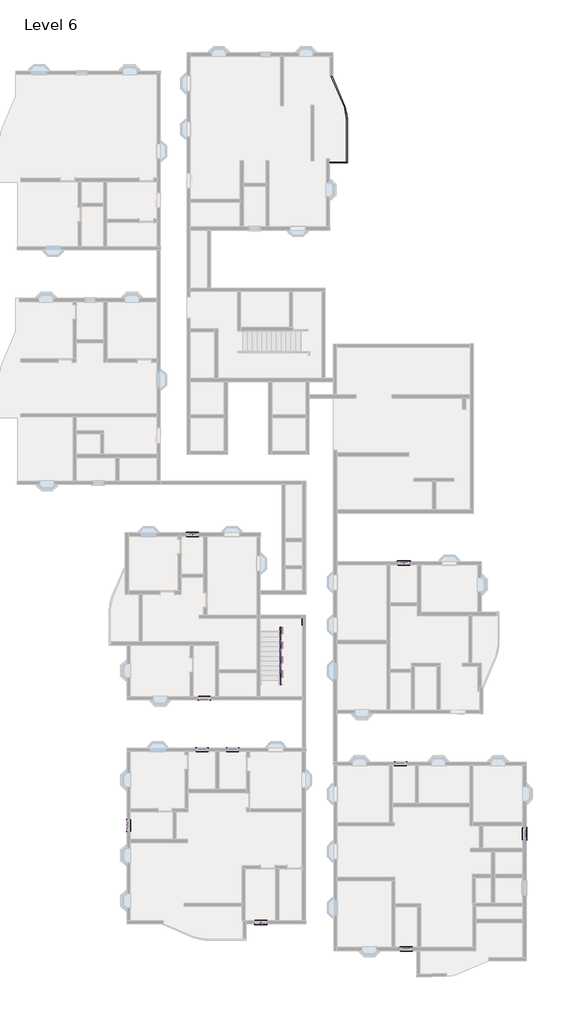
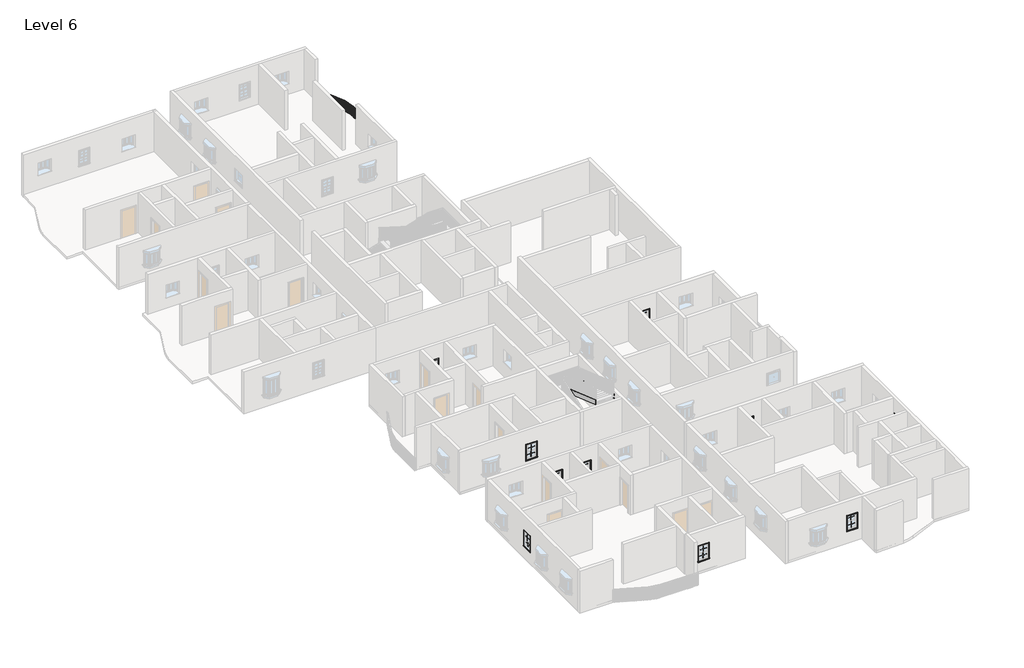
# One storey, part 13 of 14: 40 proxies, 6 members, 1 railing.
"""IFC4 building model written with IfcOpenShell, lengths in millimetres."""

from ifc_helpers import new_model, si_unit, frame, origin, place, context, project, spatial, polyline, circle_curve, outline, extrude, transform, mapped, element, save
from ifc_brep_helpers import plane_surface, cylinder_surface, revolved_surface, advanced_brep
from components import muntin_pattern_2x2_muntin_pattern_2x2_c35c595f, trim_window_exterior_flat_with_sill_e38017c9, trim_window_interior_flat_picture_frame_d728ed12

model = new_model("IFC4")

# Units and contexts
model_context = context("Model", 3, world=origin())
ifc_project = project(units=[si_unit("LENGTHUNIT", "METRE", prefix="MILLI")], contexts=[model_context])

# Site, building, storey
site = spatial("IfcSite", under=ifc_project)
building = spatial("IfcBuilding", under=site)
storey = spatial("IfcBuildingStorey", under=building, Name="Level 6", Elevation=15240.0)

# Proxies
placement = place(None, origin())
muntin_pattern_2x2_muntin_pattern_2x2_shape = muntin_pattern_2x2_muntin_pattern_2x2_c35c595f(model_context)
element("IfcBuildingElementProxy", 1, Name="Muntin Pattern_2x2 : Muntin Pattern_2x2", ObjectType="Muntin Pattern_2x2 : Muntin Pattern_2x2", at=placement, inside=storey, context=model_context, shape_type="MappedRepresentation", body=[
    mapped(muntin_pattern_2x2_muntin_pattern_2x2_shape, transform((-8150.287215, -357.5666506, 16710.025), x_axis=(1.0, 0.0, 0.0), y_axis=(0.0, 1.0, 0.0), z_axis=(0.0, 0.0, 1.0))),
])
element("IfcBuildingElementProxy", 2, Name="Muntin Pattern_2x2 : Muntin Pattern_2x2", ObjectType="Muntin Pattern_2x2 : Muntin Pattern_2x2", at=placement, inside=storey, context=model_context, shape_type="MappedRepresentation", body=[
    mapped(muntin_pattern_2x2_muntin_pattern_2x2_shape, transform((-8150.287215, -402.0166506, 16230.6), x_axis=(1.0, 0.0, 0.0), y_axis=(0.0, 1.0, 0.0), z_axis=(0.0, 0.0, 1.0))),
])
element("IfcBuildingElementProxy", 3, Name="Muntin Pattern_2x2 : Muntin Pattern_2x2", ObjectType="Muntin Pattern_2x2 : Muntin Pattern_2x2", at=placement, inside=storey, context=model_context, shape_type="MappedRepresentation", body=[
    mapped(muntin_pattern_2x2_muntin_pattern_2x2_shape, transform((-7397.812215, -10854.1166506, 16710.025), x_axis=(-1.0, 0.0, 0.0), y_axis=(0.0, -1.0, 0.0), z_axis=(0.0, 0.0, 1.0))),
])
element("IfcBuildingElementProxy", 4, Name="Muntin Pattern_2x2 : Muntin Pattern_2x2", ObjectType="Muntin Pattern_2x2 : Muntin Pattern_2x2", at=placement, inside=storey, context=model_context, shape_type="MappedRepresentation", body=[
    mapped(muntin_pattern_2x2_muntin_pattern_2x2_shape, transform((-7397.812215, -10809.6666506, 16230.6), x_axis=(-1.0, 0.0, 0.0), y_axis=(0.0, -1.0, 0.0), z_axis=(0.0, 0.0, 1.0))),
])
element("IfcBuildingElementProxy", 5, Name="Muntin Pattern_2x2 : Muntin Pattern_2x2", ObjectType="Muntin Pattern_2x2 : Muntin Pattern_2x2", at=placement, inside=storey, context=model_context, shape_type="MappedRepresentation", body=[
    mapped(muntin_pattern_2x2_muntin_pattern_2x2_shape, transform((-7540.687215, -13997.3666506, 16710.025), x_axis=(1.0, 0.0, 0.0), y_axis=(0.0, 1.0, 0.0), z_axis=(0.0, 0.0, 1.0))),
])
element("IfcBuildingElementProxy", 6, Name="Muntin Pattern_2x2 : Muntin Pattern_2x2", ObjectType="Muntin Pattern_2x2 : Muntin Pattern_2x2", at=placement, inside=storey, context=model_context, shape_type="MappedRepresentation", body=[
    mapped(muntin_pattern_2x2_muntin_pattern_2x2_shape, transform((-7540.687215, -14041.8166506, 16230.6), x_axis=(1.0, 0.0, 0.0), y_axis=(0.0, 1.0, 0.0), z_axis=(0.0, 0.0, 1.0))),
])
element("IfcBuildingElementProxy", 7, Name="Muntin Pattern_2x2 : Muntin Pattern_2x2", ObjectType="Muntin Pattern_2x2 : Muntin Pattern_2x2", at=placement, inside=storey, context=model_context, shape_type="MappedRepresentation", body=[
    mapped(muntin_pattern_2x2_muntin_pattern_2x2_shape, transform((-5597.587215, -13997.3666506, 16710.025), x_axis=(1.0, 0.0, 0.0), y_axis=(0.0, 1.0, 0.0), z_axis=(0.0, 0.0, 1.0))),
])
element("IfcBuildingElementProxy", 8, Name="Muntin Pattern_2x2 : Muntin Pattern_2x2", ObjectType="Muntin Pattern_2x2 : Muntin Pattern_2x2", at=placement, inside=storey, context=model_context, shape_type="MappedRepresentation", body=[
    mapped(muntin_pattern_2x2_muntin_pattern_2x2_shape, transform((-5597.587215, -14041.8166506, 16230.6), x_axis=(1.0, 0.0, 0.0), y_axis=(0.0, 1.0, 0.0), z_axis=(0.0, 0.0, 1.0))),
])
element("IfcBuildingElementProxy", 9, Name="Muntin Pattern_2x2 : Muntin Pattern_2x2", ObjectType="Muntin Pattern_2x2 : Muntin Pattern_2x2", at=placement, inside=storey, context=model_context, shape_type="MappedRepresentation", body=[
    mapped(muntin_pattern_2x2_muntin_pattern_2x2_shape, transform((-12255.562215, -18863.6994419, 16710.025), x_axis=(0.0, 1.0, 0.0), y_axis=(-1.0, 0.0, 0.0), z_axis=(0.0, 0.0, 1.0))),
])
element("IfcBuildingElementProxy", 10, Name="Muntin Pattern_2x2 : Muntin Pattern_2x2", ObjectType="Muntin Pattern_2x2 : Muntin Pattern_2x2", at=placement, inside=storey, context=model_context, shape_type="MappedRepresentation", body=[
    mapped(muntin_pattern_2x2_muntin_pattern_2x2_shape, transform((-12211.112215, -18863.6994419, 16230.6), x_axis=(0.0, 1.0, 0.0), y_axis=(-1.0, 0.0, 0.0), z_axis=(0.0, 0.0, 1.0))),
])
element("IfcBuildingElementProxy", 11, Name="Muntin Pattern_2x2 : Muntin Pattern_2x2", ObjectType="Muntin Pattern_2x2 : Muntin Pattern_2x2", at=placement, inside=storey, context=model_context, shape_type="MappedRepresentation", body=[
    mapped(muntin_pattern_2x2_muntin_pattern_2x2_shape, transform((-3806.2891351, -25065.4166506, 16710.025), x_axis=(-1.0, 0.0, 0.0), y_axis=(0.0, -1.0, 0.0), z_axis=(0.0, 0.0, 1.0))),
])
element("IfcBuildingElementProxy", 12, Name="Muntin Pattern_2x2 : Muntin Pattern_2x2", ObjectType="Muntin Pattern_2x2 : Muntin Pattern_2x2", at=placement, inside=storey, context=model_context, shape_type="MappedRepresentation", body=[
    mapped(muntin_pattern_2x2_muntin_pattern_2x2_shape, transform((-3806.2891351, -25020.9666506, 16230.6), x_axis=(-1.0, 0.0, 0.0), y_axis=(0.0, -1.0, 0.0), z_axis=(0.0, 0.0, 1.0))),
])
element("IfcBuildingElementProxy", 13, Name="Muntin Pattern_2x2 : Muntin Pattern_2x2", ObjectType="Muntin Pattern_2x2 : Muntin Pattern_2x2", at=placement, inside=storey, context=model_context, shape_type="MappedRepresentation", body=[
    mapped(muntin_pattern_2x2_muntin_pattern_2x2_shape, transform((5410.0380523, -26615.6292694, 16710.025), x_axis=(1.0, 0.0, 0.0), y_axis=(0.0, 1.0, 0.0), z_axis=(0.0, 0.0, 1.0))),
])
element("IfcBuildingElementProxy", 14, Name="Muntin Pattern_2x2 : Muntin Pattern_2x2", ObjectType="Muntin Pattern_2x2 : Muntin Pattern_2x2", at=placement, inside=storey, context=model_context, shape_type="MappedRepresentation", body=[
    mapped(muntin_pattern_2x2_muntin_pattern_2x2_shape, transform((5410.0380523, -26660.0792694, 16230.6), x_axis=(1.0, 0.0, 0.0), y_axis=(0.0, 1.0, 0.0), z_axis=(0.0, 0.0, 1.0))),
])
element("IfcBuildingElementProxy", 15, Name="Muntin Pattern_2x2 : Muntin Pattern_2x2", ObjectType="Muntin Pattern_2x2 : Muntin Pattern_2x2", at=placement, inside=storey, context=model_context, shape_type="MappedRepresentation", body=[
    mapped(muntin_pattern_2x2_muntin_pattern_2x2_shape, transform((12982.4130523, -19379.8042694, 16710.025), x_axis=(0.0, -1.0, 0.0), y_axis=(1.0, 0.0, 0.0), z_axis=(0.0, 0.0, 1.0))),
])
element("IfcBuildingElementProxy", 16, Name="Muntin Pattern_2x2 : Muntin Pattern_2x2", ObjectType="Muntin Pattern_2x2 : Muntin Pattern_2x2", at=placement, inside=storey, context=model_context, shape_type="MappedRepresentation", body=[
    mapped(muntin_pattern_2x2_muntin_pattern_2x2_shape, transform((12937.9630523, -19379.8042694, 16230.6), x_axis=(0.0, -1.0, 0.0), y_axis=(1.0, 0.0, 0.0), z_axis=(0.0, 0.0, 1.0))),
])
element("IfcBuildingElementProxy", 17, Name="Muntin Pattern_2x2 : Muntin Pattern_2x2", ObjectType="Muntin Pattern_2x2 : Muntin Pattern_2x2", at=placement, inside=storey, context=model_context, shape_type="MappedRepresentation", body=[
    mapped(muntin_pattern_2x2_muntin_pattern_2x2_shape, transform((5048.0880523, -14880.8292694, 16710.025), x_axis=(1.0, 0.0, 0.0), y_axis=(0.0, 1.0, 0.0), z_axis=(0.0, 0.0, 1.0))),
])
element("IfcBuildingElementProxy", 18, Name="Muntin Pattern_2x2 : Muntin Pattern_2x2", ObjectType="Muntin Pattern_2x2 : Muntin Pattern_2x2", at=placement, inside=storey, context=model_context, shape_type="MappedRepresentation", body=[
    mapped(muntin_pattern_2x2_muntin_pattern_2x2_shape, transform((5048.0880523, -14925.2792694, 16230.6), x_axis=(1.0, 0.0, 0.0), y_axis=(0.0, 1.0, 0.0), z_axis=(0.0, 0.0, 1.0))),
])
element("IfcBuildingElementProxy", 19, Name="Muntin Pattern_2x2 : Muntin Pattern_2x2", ObjectType="Muntin Pattern_2x2 : Muntin Pattern_2x2", at=placement, inside=storey, context=model_context, shape_type="MappedRepresentation", body=[
    mapped(muntin_pattern_2x2_muntin_pattern_2x2_shape, transform((5257.6380523, -2168.1292694, 16710.025), x_axis=(1.0, 0.0, 0.0), y_axis=(0.0, 1.0, 0.0), z_axis=(0.0, 0.0, 1.0))),
])
element("IfcBuildingElementProxy", 20, Name="Muntin Pattern_2x2 : Muntin Pattern_2x2", ObjectType="Muntin Pattern_2x2 : Muntin Pattern_2x2", at=placement, inside=storey, context=model_context, shape_type="MappedRepresentation", body=[
    mapped(muntin_pattern_2x2_muntin_pattern_2x2_shape, transform((5257.6380523, -2212.5792694, 16230.6), x_axis=(1.0, 0.0, 0.0), y_axis=(0.0, 1.0, 0.0), z_axis=(0.0, 0.0, 1.0))),
])
trim_window_exterior_flat_with_sill_shape = trim_window_exterior_flat_with_sill_e38017c9(model_context)
element("IfcBuildingElementProxy", 21, Name="Trim-Window-Exterior-Flat : with Sill", ObjectType="Trim-Window-Exterior-Flat : with Sill", at=placement, inside=storey, context=model_context, shape_type="MappedRepresentation", body=[
    mapped(trim_window_exterior_flat_with_sill_shape, transform((-8150.287215, -322.6416506, 17221.2), x_axis=(-1.0, 0.0, 0.0), y_axis=(0.0, 0.0, 1.0), z_axis=(0.0, 1.0, 0.0))),
])
element("IfcBuildingElementProxy", 22, Name="Trim-Window-Exterior-Flat : with Sill", ObjectType="Trim-Window-Exterior-Flat : with Sill", at=placement, inside=storey, context=model_context, shape_type="MappedRepresentation", body=[
    mapped(trim_window_exterior_flat_with_sill_shape, transform((-7397.812215, -10889.0416506, 17221.2), x_axis=(1.0, 0.0, 0.0), y_axis=(0.0, 0.0, 1.0), z_axis=(0.0, -1.0, 0.0))),
])
element("IfcBuildingElementProxy", 23, Name="Trim-Window-Exterior-Flat : with Sill", ObjectType="Trim-Window-Exterior-Flat : with Sill", at=placement, inside=storey, context=model_context, shape_type="MappedRepresentation", body=[
    mapped(trim_window_exterior_flat_with_sill_shape, transform((-7540.687215, -13962.4416506, 17221.2), x_axis=(-1.0, 0.0, 0.0), y_axis=(0.0, 0.0, 1.0), z_axis=(0.0, 1.0, 0.0))),
])
element("IfcBuildingElementProxy", 24, Name="Trim-Window-Exterior-Flat : with Sill", ObjectType="Trim-Window-Exterior-Flat : with Sill", at=placement, inside=storey, context=model_context, shape_type="MappedRepresentation", body=[
    mapped(trim_window_exterior_flat_with_sill_shape, transform((-5597.587215, -13962.4416506, 17221.2), x_axis=(-1.0, 0.0, 0.0), y_axis=(0.0, 0.0, 1.0), z_axis=(0.0, 1.0, 0.0))),
])
element("IfcBuildingElementProxy", 25, Name="Trim-Window-Exterior-Flat : with Sill", ObjectType="Trim-Window-Exterior-Flat : with Sill", at=placement, inside=storey, context=model_context, shape_type="MappedRepresentation", body=[
    mapped(trim_window_exterior_flat_with_sill_shape, transform((-12290.487215, -18863.6994419, 17221.2), x_axis=(0.0, -1.0, 0.0), y_axis=(0.0, 0.0, 1.0), z_axis=(-1.0, 0.0, 0.0))),
])
element("IfcBuildingElementProxy", 26, Name="Trim-Window-Exterior-Flat : with Sill", ObjectType="Trim-Window-Exterior-Flat : with Sill", at=placement, inside=storey, context=model_context, shape_type="MappedRepresentation", body=[
    mapped(trim_window_exterior_flat_with_sill_shape, transform((-3806.2891351, -25100.3416506, 17221.2), x_axis=(1.0, 0.0, 0.0), y_axis=(0.0, 0.0, 1.0), z_axis=(0.0, -1.0, 0.0))),
])
element("IfcBuildingElementProxy", 27, Name="Trim-Window-Exterior-Flat : with Sill", ObjectType="Trim-Window-Exterior-Flat : with Sill", at=placement, inside=storey, context=model_context, shape_type="MappedRepresentation", body=[
    mapped(trim_window_exterior_flat_with_sill_shape, transform((5410.0380523, -26580.7042694, 17221.2), x_axis=(-1.0, 0.0, 0.0), y_axis=(0.0, 0.0, 1.0), z_axis=(0.0, 1.0, 0.0))),
])
element("IfcBuildingElementProxy", 28, Name="Trim-Window-Exterior-Flat : with Sill", ObjectType="Trim-Window-Exterior-Flat : with Sill", at=placement, inside=storey, context=model_context, shape_type="MappedRepresentation", body=[
    mapped(trim_window_exterior_flat_with_sill_shape, transform((13017.3380523, -19379.8042694, 17221.2), x_axis=(0.0, 1.0, 0.0), y_axis=(0.0, 0.0, 1.0), z_axis=(1.0, 0.0, 0.0))),
])
element("IfcBuildingElementProxy", 29, Name="Trim-Window-Exterior-Flat : with Sill", ObjectType="Trim-Window-Exterior-Flat : with Sill", at=placement, inside=storey, context=model_context, shape_type="MappedRepresentation", body=[
    mapped(trim_window_exterior_flat_with_sill_shape, transform((5048.0880523, -14845.9042694, 17221.2), x_axis=(-1.0, 0.0, 0.0), y_axis=(0.0, 0.0, 1.0), z_axis=(0.0, 1.0, 0.0))),
])
element("IfcBuildingElementProxy", 30, Name="Trim-Window-Exterior-Flat : with Sill", ObjectType="Trim-Window-Exterior-Flat : with Sill", at=placement, inside=storey, context=model_context, shape_type="MappedRepresentation", body=[
    mapped(trim_window_exterior_flat_with_sill_shape, transform((5257.6380523, -2133.2042694, 17221.2), x_axis=(-1.0, 0.0, 0.0), y_axis=(0.0, 0.0, 1.0), z_axis=(0.0, 1.0, 0.0))),
])
trim_window_interior_flat_picture_frame_shape = trim_window_interior_flat_picture_frame_d728ed12(model_context)
element("IfcBuildingElementProxy", 31, Name="Trim-Window-Interior-Flat : Picture Frame", ObjectType="Trim-Window-Interior-Flat : Picture Frame", at=placement, inside=storey, context=model_context, shape_type="MappedRepresentation", body=[
    mapped(trim_window_interior_flat_picture_frame_shape, transform((-8150.287215, -525.8416506, 17221.2), x_axis=(1.0, 0.0, 0.0), y_axis=(0.0, 0.0, 1.0), z_axis=(0.0, -1.0, 0.0))),
])
element("IfcBuildingElementProxy", 32, Name="Trim-Window-Interior-Flat : Picture Frame", ObjectType="Trim-Window-Interior-Flat : Picture Frame", at=placement, inside=storey, context=model_context, shape_type="MappedRepresentation", body=[
    mapped(trim_window_interior_flat_picture_frame_shape, transform((-7397.812215, -10685.8416506, 17221.2), x_axis=(-1.0, 0.0, 0.0), y_axis=(0.0, 0.0, 1.0), z_axis=(0.0, 1.0, 0.0))),
])
element("IfcBuildingElementProxy", 33, Name="Trim-Window-Interior-Flat : Picture Frame", ObjectType="Trim-Window-Interior-Flat : Picture Frame", at=placement, inside=storey, context=model_context, shape_type="MappedRepresentation", body=[
    mapped(trim_window_interior_flat_picture_frame_shape, transform((-7540.687215, -14165.6416506, 17221.2), x_axis=(1.0, 0.0, 0.0), y_axis=(0.0, 0.0, 1.0), z_axis=(0.0, -1.0, 0.0))),
])
element("IfcBuildingElementProxy", 34, Name="Trim-Window-Interior-Flat : Picture Frame", ObjectType="Trim-Window-Interior-Flat : Picture Frame", at=placement, inside=storey, context=model_context, shape_type="MappedRepresentation", body=[
    mapped(trim_window_interior_flat_picture_frame_shape, transform((-5597.587215, -14165.6416506, 17221.2), x_axis=(1.0, 0.0, 0.0), y_axis=(0.0, 0.0, 1.0), z_axis=(0.0, -1.0, 0.0))),
])
element("IfcBuildingElementProxy", 35, Name="Trim-Window-Interior-Flat : Picture Frame", ObjectType="Trim-Window-Interior-Flat : Picture Frame", at=placement, inside=storey, context=model_context, shape_type="MappedRepresentation", body=[
    mapped(trim_window_interior_flat_picture_frame_shape, transform((-12087.287215, -18863.6994419, 17221.2), x_axis=(0.0, 1.0, 0.0), y_axis=(0.0, 0.0, 1.0), z_axis=(1.0, 0.0, 0.0))),
])
element("IfcBuildingElementProxy", 36, Name="Trim-Window-Interior-Flat : Picture Frame", ObjectType="Trim-Window-Interior-Flat : Picture Frame", at=placement, inside=storey, context=model_context, shape_type="MappedRepresentation", body=[
    mapped(trim_window_interior_flat_picture_frame_shape, transform((-3806.2891351, -24897.1416506, 17221.2), x_axis=(-1.0, 0.0, 0.0), y_axis=(0.0, 0.0, 1.0), z_axis=(0.0, 1.0, 0.0))),
])
element("IfcBuildingElementProxy", 37, Name="Trim-Window-Interior-Flat : Picture Frame", ObjectType="Trim-Window-Interior-Flat : Picture Frame", at=placement, inside=storey, context=model_context, shape_type="MappedRepresentation", body=[
    mapped(trim_window_interior_flat_picture_frame_shape, transform((5410.0380523, -26783.9042694, 17221.2), x_axis=(1.0, 0.0, 0.0), y_axis=(0.0, 0.0, 1.0), z_axis=(0.0, -1.0, 0.0))),
])
element("IfcBuildingElementProxy", 38, Name="Trim-Window-Interior-Flat : Picture Frame", ObjectType="Trim-Window-Interior-Flat : Picture Frame", at=placement, inside=storey, context=model_context, shape_type="MappedRepresentation", body=[
    mapped(trim_window_interior_flat_picture_frame_shape, transform((12814.1380523, -19379.8042694, 17221.2), x_axis=(0.0, -1.0, 0.0), y_axis=(0.0, 0.0, 1.0), z_axis=(-1.0, 0.0, 0.0))),
])
element("IfcBuildingElementProxy", 39, Name="Trim-Window-Interior-Flat : Picture Frame", ObjectType="Trim-Window-Interior-Flat : Picture Frame", at=placement, inside=storey, context=model_context, shape_type="MappedRepresentation", body=[
    mapped(trim_window_interior_flat_picture_frame_shape, transform((5048.0880523, -15049.1042694, 17221.2), x_axis=(1.0, 0.0, 0.0), y_axis=(0.0, 0.0, 1.0), z_axis=(0.0, -1.0, 0.0))),
])
element("IfcBuildingElementProxy", 40, Name="Trim-Window-Interior-Flat : Picture Frame", ObjectType="Trim-Window-Interior-Flat : Picture Frame", at=placement, inside=storey, context=model_context, shape_type="MappedRepresentation", body=[
    mapped(trim_window_interior_flat_picture_frame_shape, transform((5257.6380523, -2336.4042694, 17221.2), x_axis=(1.0, 0.0, 0.0), y_axis=(0.0, 0.0, 1.0), z_axis=(0.0, -1.0, 0.0))),
])

# Members
element("IfcMember", 41, ObjectType="Stringer - 2\" Width", at=placement, inside=storey, context=model_context, shape_type="SweptSolid", body=[
    extrude(outline(polyline([(-9955.5916506, 15240.0), (-9955.5916506, 15431.3592169), (-6325.8738327, 16687.8), (-5713.7916506, 16687.8), (-5713.7916506, 16577.1301656), (-9576.612129, 15240.0), (-9955.5916506, 15240.0)])), frame((-3908.487215, 0.0, 0.0), z_axis=(1.0, 0.0, 0.0), x_axis=(0.0, 1.0, 0.0)), (0.0, 0.0, 1.0), 50.8),
])
element("IfcMember", 42, ObjectType="Stringer - 2\" Width", at=placement, inside=storey, context=model_context, shape_type="SweptSolid", body=[
    extrude(outline(polyline([(-3908.487215, -5713.7916506), (-3908.487215, -5662.9916506), (-1190.687215, -5662.9916506), (-1190.687215, -5713.7916506), (-3908.487215, -5713.7916506)])), frame((0.0, 0.0, 16383.0), z_axis=(0.0, 0.0, 1.0), x_axis=(1.0, 0.0, 0.0)), (0.0, 0.0, 1.0), 304.8),
])
element("IfcMember", 43, ObjectType="Stringer - 2\" Width", at=placement, inside=storey, context=model_context, shape_type="SweptSolid", body=[
    extrude(outline(polyline([(-5662.9916506, 16587.5476784), (-5662.9916506, 16383.0), (-6003.8711722, 16383.0), (-9949.2416506, 17748.7051656), (-9949.2416506, 18071.2496015), (-5662.9916506, 16587.5476784)])), frame((-1190.687215, 0.0, 0.0), z_axis=(1.0, 0.0, 0.0), x_axis=(0.0, 1.0, 0.0)), (0.0, 0.0, 1.0), 50.8),
])
element("IfcMember", 44, ObjectType="Stringer - 2\" Width", at=placement, inside=storey, context=model_context, shape_type="SweptSolid", body=[
    extrude(outline(polyline([(-9955.5916506, 15240.0), (-9955.5916506, 15431.3592169), (-6342.4416506, 16682.0649861), (-6342.4416506, 16359.5205502), (-9576.612129, 15240.0), (-9955.5916506, 15240.0)])), frame((-2593.7381751, 0.0, 0.0), z_axis=(1.0, 0.0, 0.0), x_axis=(0.0, 1.0, 0.0)), (0.0, 0.0, 1.0), 50.8),
])
element("IfcMember", 45, ObjectType="Stringer - 2\" Width", at=placement, inside=storey, context=model_context, shape_type="SweptSolid", body=[
    extrude(outline(polyline([(-2593.7381751, -6342.4416506), (-2593.7381751, -6291.6416506), (-2492.1381751, -6291.6416506), (-2492.1381751, -6342.4416506), (-2593.7381751, -6342.4416506)])), frame((0.0, 0.0, 16383.0), z_axis=(0.0, 0.0, 1.0), x_axis=(1.0, 0.0, 0.0)), (0.0, 0.0, 1.0), 304.8),
])
element("IfcMember", 46, ObjectType="Stringer - 2\" Width", at=placement, inside=storey, context=model_context, shape_type="SweptSolid", body=[
    extrude(outline(polyline([(-6291.6416506, 16805.1572938), (-6291.6416506, 16482.6128579), (-9949.2416506, 17748.7051656), (-9949.2416506, 18071.2496015), (-6291.6416506, 16805.1572938)])), frame((-2492.1381751, 0.0, 0.0), z_axis=(1.0, 0.0, 0.0), x_axis=(0.0, 1.0, 0.0)), (0.0, 0.0, 1.0), 50.8),
])

# Railing
element("IfcRailing", 47, ObjectType="Handrail - Rectangular", at=placement, inside=storey, context=model_context, shape_type="SolidModel", body=[
    advanced_brep(
    [(549.8108649, 23180.4215905, 16154.4), (549.8108649, 23180.4215905, 16103.6), (549.8108649, 23129.6215905, 16103.6), (549.8108649, 23129.6215905, 16154.4), (1629.3108649, 23180.4215905, 16154.4), (1629.3108649, 23180.4215905, 16103.6), (1680.1108649, 23129.6215905, 16103.6), (1680.1108649, 23129.6215905, 16154.4), (1629.3108649, 25921.9580583, 16154.4), (1629.3108649, 25921.9580583, 16103.6), (1680.1108649, 25921.9580583, 16103.6), (1680.1108649, 25921.9580583, 16154.4), (1475.5051478, 26671.8537734, 16103.6), (1475.5051478, 26671.8537734, 16154.4), (1522.203662, 26691.8509925, 16103.6), (1522.203662, 26691.8509925, 16154.4), (640.7616078, 28621.188975, 16154.4), (687.460122, 28641.186194, 16154.4), (687.460122, 28641.186194, 16103.6), (640.7616078, 28621.188975, 16103.6)],
    [
        (0, 1),
        (1, 2),
        (2, 3),
        (3, 0),
        (0, 4),
        (4, 5),
        (5, 1),
        (5, 6),
        (6, 2),
        (6, 7),
        (7, 3),
        (7, 4),
        (4, 8),
        (8, 9),
        (9, 5),
        (9, 10),
        (10, 6),
        (10, 11),
        (11, 7),
        (11, 8),
        (12, 9, circle_curve(frame((-275.6891351, 25921.9580583, 16103.6), z_axis=(0.0, 0.0, -1.0), x_axis=(1.0, 0.0, 0.0)), 1905.0)),
        (8, 13, circle_curve(frame((-275.6891351, 25921.9580583, 16154.4), z_axis=(0.0, 0.0, 1.0), x_axis=(1.0, 0.0, 0.0)), 1905.0)),
        (13, 12),
        (14, 10, circle_curve(frame((-275.6891351, 25921.9580583, 16103.6), z_axis=(0.0, 0.0, -1.0), x_axis=(1.0, 0.0, 0.0)), 1955.8)),
        (12, 14),
        (15, 11, circle_curve(frame((-275.6891351, 25921.9580583, 16154.4), z_axis=(0.0, 0.0, -1.0), x_axis=(1.0, 0.0, 0.0)), 1955.8)),
        (14, 15),
        (15, 13),
        (16, 17),
        (17, 18),
        (18, 19),
        (19, 16),
        (13, 16),
        (19, 12),
        (18, 14),
        (17, 15),
    ],
    [
        plane_surface(frame((549.8108649, 23155.0215905, 16154.4), z_axis=(-1.0, 0.0, 0.0), x_axis=(0.0, 1.0, 0.0))),
        plane_surface(frame((549.8108649, 23180.4215905, 16154.4), z_axis=(0.0, 1.0, 0.0), x_axis=(1.0, 0.0, 0.0))),
        plane_surface(frame((549.8108649, 23180.4215905, 16103.6), z_axis=(0.0, 0.0, -1.0), x_axis=(1.0, 0.0, 0.0))),
        plane_surface(frame((549.8108649, 23129.6215905, 16103.6), z_axis=(0.0, -1.0, 0.0), x_axis=(1.0, 0.0, 0.0))),
        plane_surface(frame((549.8108649, 23129.6215905, 16154.4), z_axis=(0.0, 0.0, 1.0), x_axis=(1.0, 0.0, 0.0))),
        plane_surface(frame((1629.3108649, 23180.4215905, 16154.4), z_axis=(-1.0, 0.0, 0.0), x_axis=(0.0, 1.0, 0.0))),
        plane_surface(frame((1629.3108649, 23180.4215905, 16103.6), z_axis=(0.0, 0.0, -1.0), x_axis=(0.0, 1.0, 0.0))),
        plane_surface(frame((1680.1108649, 23129.6215905, 16103.6), z_axis=(1.0, 0.0, 0.0), x_axis=(0.0, 1.0, 0.0))),
        plane_surface(frame((1680.1108649, 23129.6215905, 16154.4), z_axis=(0.0, 0.0, 1.0), x_axis=(0.0, 1.0, 0.0))),
        revolved_surface(polyline([(1629.3108649, 25921.9580583, 16154.4), (1629.3108649, 25921.9580583, 16103.6)]), (-275.6891351, 25921.9580583, 16154.4), (0.0, 0.0, 1.0)),
        plane_surface(frame((-275.6891351, 25921.9580583, 16103.6), z_axis=(0.0, 0.0, -1.0), x_axis=(1.0, 0.0, 0.0))),
        cylinder_surface(frame((-275.6891351, 25921.9580583, 16154.4), z_axis=(0.0, 0.0, 1.0), x_axis=(1.0, 0.0, 0.0)), 1955.8),
        plane_surface(frame((-275.6891351, 25921.9580583, 16154.4), z_axis=(0.0, 0.0, 1.0), x_axis=(1.0, 0.0, 0.0))),
        plane_surface(frame((664.1108649, 28631.1875845, 16154.4), z_axis=(-0.39364604467361036, 0.91926209076238, 0.0), x_axis=(0.91926209076238, 0.39364604467361036, 0.0))),
        plane_surface(frame((1475.5051478, 26671.8537734, 16154.4), z_axis=(-0.91926209076238, -0.3936460446736102, 0.0), x_axis=(-0.3936460446736102, 0.91926209076238, 0.0))),
        plane_surface(frame((1475.5051478, 26671.8537734, 16103.6), z_axis=(0.0, 0.0, -1.0), x_axis=(-0.3936460446736102, 0.91926209076238, 0.0))),
        plane_surface(frame((1522.203662, 26691.8509925, 16103.6), z_axis=(0.91926209076238, 0.3936460446736102, 0.0), x_axis=(-0.3936460446736102, 0.91926209076238, 0.0))),
        plane_surface(frame((1522.203662, 26691.8509925, 16154.4), z_axis=(0.0, 0.0, 1.0), x_axis=(-0.3936460446736102, 0.91926209076238, 0.0))),
    ],
    [
        (0, [[1, 2, 3, 4]]),
        (1, [[-1, 5, 6, 7]]),
        (2, [[-2, -7, 8, 9]]),
        (3, [[-3, -9, 10, 11]]),
        (4, [[-4, -11, 12, -5]]),
        (5, [[-6, 13, 14, 15]]),
        (6, [[-8, -15, 16, 17]]),
        (7, [[-10, -17, 18, 19]]),
        (8, [[-12, -19, 20, -13]]),
        (9, [[21, -14, 22, 23]]),
        (10, [[24, -16, -21, 25]]),
        (11, [[26, -18, -24, 27]]),
        (12, [[-22, -20, -26, 28]]),
        (13, [[29, 30, 31, 32]]),
        (14, [[-23, 33, -32, 34]]),
        (15, [[-25, -34, -31, 35]]),
        (16, [[-27, -35, -30, 36]]),
        (17, [[-28, -36, -29, -33]]),
    ],
),
    extrude(outline(polyline([(711.4710921, 28544.7864585), (693.9591493, 28537.2875014), (686.4601921, 28554.7994442), (703.9721349, 28562.2984014), (711.4710921, 28544.7864585)])), frame((0.0, 0.0, 15240.0), z_axis=(0.0, 0.0, 1.0), x_axis=(1.0, 0.0, 0.0)), (0.0, 0.0, 1.0), 863.6),
    extrude(outline(polyline([(751.4655302, 28451.3894301), (733.9535874, 28443.890473), (726.4546303, 28461.4024158), (743.9665731, 28468.9013729), (751.4655302, 28451.3894301)])), frame((0.0, 0.0, 15240.0), z_axis=(0.0, 0.0, 1.0), x_axis=(1.0, 0.0, 0.0)), (0.0, 0.0, 1.0), 863.6),
    extrude(outline(polyline([(791.4599684, 28357.9924017), (773.9480255, 28350.4934445), (766.4490684, 28368.0053874), (783.9610112, 28375.5043445), (791.4599684, 28357.9924017)])), frame((0.0, 0.0, 15240.0), z_axis=(0.0, 0.0, 1.0), x_axis=(1.0, 0.0, 0.0)), (0.0, 0.0, 1.0), 863.6),
    extrude(outline(polyline([(831.4544065, 28264.5953733), (813.9424637, 28257.0964161), (806.4435065, 28274.608359), (823.9554494, 28282.1073161), (831.4544065, 28264.5953733)])), frame((0.0, 0.0, 15240.0), z_axis=(0.0, 0.0, 1.0), x_axis=(1.0, 0.0, 0.0)), (0.0, 0.0, 1.0), 863.6),
    extrude(outline(polyline([(871.4488446, 28171.1983449), (853.9369018, 28163.6993877), (846.4379447, 28181.2113305), (863.9498875, 28188.7102877), (871.4488446, 28171.1983449)])), frame((0.0, 0.0, 15240.0), z_axis=(0.0, 0.0, 1.0), x_axis=(1.0, 0.0, 0.0)), (0.0, 0.0, 1.0), 863.6),
    extrude(outline(polyline([(911.4432828, 28077.8013164), (893.93134, 28070.3023593), (886.4323828, 28087.8143021), (903.9443256, 28095.3132593), (911.4432828, 28077.8013164)])), frame((0.0, 0.0, 15240.0), z_axis=(0.0, 0.0, 1.0), x_axis=(1.0, 0.0, 0.0)), (0.0, 0.0, 1.0), 863.6),
    extrude(outline(polyline([(951.4377209, 27984.404288), (933.9257781, 27976.9053309), (926.4268209, 27994.4172737), (943.9387638, 28001.9162308), (951.4377209, 27984.404288)])), frame((0.0, 0.0, 15240.0), z_axis=(0.0, 0.0, 1.0), x_axis=(1.0, 0.0, 0.0)), (0.0, 0.0, 1.0), 863.6),
    extrude(outline(polyline([(991.4321591, 27891.0072596), (973.9202162, 27883.5083024), (966.4212591, 27901.0202453), (983.9332019, 27908.5192024), (991.4321591, 27891.0072596)])), frame((0.0, 0.0, 15240.0), z_axis=(0.0, 0.0, 1.0), x_axis=(1.0, 0.0, 0.0)), (0.0, 0.0, 1.0), 863.6),
    extrude(outline(polyline([(1031.4265972, 27797.6102312), (1013.9146544, 27790.111274), (1006.4156972, 27807.6232168), (1023.9276401, 27815.122174), (1031.4265972, 27797.6102312)])), frame((0.0, 0.0, 15240.0), z_axis=(0.0, 0.0, 1.0), x_axis=(1.0, 0.0, 0.0)), (0.0, 0.0, 1.0), 863.6),
    extrude(outline(polyline([(1071.4210353, 27704.2132027), (1053.9090925, 27696.7142456), (1046.4101354, 27714.2261884), (1063.9220782, 27721.7251456), (1071.4210353, 27704.2132027)])), frame((0.0, 0.0, 15240.0), z_axis=(0.0, 0.0, 1.0), x_axis=(1.0, 0.0, 0.0)), (0.0, 0.0, 1.0), 863.6),
    extrude(outline(polyline([(1111.4154735, 27610.8161743), (1093.9035307, 27603.3172172), (1086.4045735, 27620.82916), (1103.9165163, 27628.3281172), (1111.4154735, 27610.8161743)])), frame((0.0, 0.0, 15240.0), z_axis=(0.0, 0.0, 1.0), x_axis=(1.0, 0.0, 0.0)), (0.0, 0.0, 1.0), 863.6),
    extrude(outline(polyline([(1151.4099116, 27517.4191459), (1133.8979688, 27509.9201888), (1126.3990116, 27527.4321316), (1143.9109545, 27534.9310887), (1151.4099116, 27517.4191459)])), frame((0.0, 0.0, 15240.0), z_axis=(0.0, 0.0, 1.0), x_axis=(1.0, 0.0, 0.0)), (0.0, 0.0, 1.0), 863.6),
    extrude(outline(polyline([(1191.4043498, 27424.0221175), (1173.8924069, 27416.5231603), (1166.3934498, 27434.0351032), (1183.9053926, 27441.5340603), (1191.4043498, 27424.0221175)])), frame((0.0, 0.0, 15240.0), z_axis=(0.0, 0.0, 1.0), x_axis=(1.0, 0.0, 0.0)), (0.0, 0.0, 1.0), 863.6),
    extrude(outline(polyline([(1231.3987879, 27330.6250891), (1213.8868451, 27323.1261319), (1206.3878879, 27340.6380747), (1223.8998307, 27348.1370319), (1231.3987879, 27330.6250891)])), frame((0.0, 0.0, 15240.0), z_axis=(0.0, 0.0, 1.0), x_axis=(1.0, 0.0, 0.0)), (0.0, 0.0, 1.0), 863.6),
    extrude(outline(polyline([(1271.393226, 27237.2280606), (1253.8812832, 27229.7291035), (1246.3823261, 27247.2410463), (1263.8942689, 27254.7400035), (1271.393226, 27237.2280606)])), frame((0.0, 0.0, 15240.0), z_axis=(0.0, 0.0, 1.0), x_axis=(1.0, 0.0, 0.0)), (0.0, 0.0, 1.0), 863.6),
    extrude(outline(polyline([(1311.3876642, 27143.8310322), (1293.8757213, 27136.3320751), (1286.3767642, 27153.8440179), (1303.888707, 27161.342975), (1311.3876642, 27143.8310322)])), frame((0.0, 0.0, 15240.0), z_axis=(0.0, 0.0, 1.0), x_axis=(1.0, 0.0, 0.0)), (0.0, 0.0, 1.0), 863.6),
    extrude(outline(polyline([(1351.3821023, 27050.4340038), (1333.8701595, 27042.9350466), (1326.3712023, 27060.4469895), (1343.8831452, 27067.9459466), (1351.3821023, 27050.4340038)])), frame((0.0, 0.0, 15240.0), z_axis=(0.0, 0.0, 1.0), x_axis=(1.0, 0.0, 0.0)), (0.0, 0.0, 1.0), 863.6),
    extrude(outline(polyline([(1391.3765405, 26957.0369754), (1373.8645976, 26949.5380182), (1366.3656405, 26967.0499611), (1383.8775833, 26974.5489182), (1391.3765405, 26957.0369754)])), frame((0.0, 0.0, 15240.0), z_axis=(0.0, 0.0, 1.0), x_axis=(1.0, 0.0, 0.0)), (0.0, 0.0, 1.0), 863.6),
    extrude(outline(polyline([(1431.3709786, 26863.639947), (1413.8590358, 26856.1409898), (1406.3600786, 26873.6529326), (1423.8720214, 26881.1518898), (1431.3709786, 26863.639947)])), frame((0.0, 0.0, 15240.0), z_axis=(0.0, 0.0, 1.0), x_axis=(1.0, 0.0, 0.0)), (0.0, 0.0, 1.0), 863.6),
    extrude(outline(polyline([(1471.3654167, 26770.2429185), (1453.8534739, 26762.7439614), (1446.3545168, 26780.2559042), (1463.8664596, 26787.7548614), (1471.3654167, 26770.2429185)])), frame((0.0, 0.0, 15240.0), z_axis=(0.0, 0.0, 1.0), x_axis=(1.0, 0.0, 0.0)), (0.0, 0.0, 1.0), 863.6),
    extrude(outline(polyline([(1537.4917391, 26611.722401), (1519.7200483, 26604.8616791), (1512.8593263, 26622.6333699), (1530.6310171, 26629.4940918), (1537.4917391, 26611.722401)])), frame((0.0, 0.0, 15240.0), z_axis=(0.0, 0.0, 1.0), x_axis=(1.0, 0.0, 0.0)), (0.0, 0.0, 1.0), 863.6),
    extrude(outline(polyline([(1571.2676162, 26515.3807493), (1553.1596103, 26509.4644479), (1547.2433088, 26527.5724538), (1565.3513147, 26533.4887552), (1571.2676162, 26515.3807493)])), frame((0.0, 0.0, 15240.0), z_axis=(0.0, 0.0, 1.0), x_axis=(1.0, 0.0, 0.0)), (0.0, 0.0, 1.0), 863.6),
    extrude(outline(polyline([(1599.9284504, 26417.3956468), (1581.5342785, 26412.4401508), (1576.5787825, 26430.8343227), (1594.9729544, 26435.7898187), (1599.9284504, 26417.3956468)])), frame((0.0, 0.0, 15240.0), z_axis=(0.0, 0.0, 1.0), x_axis=(1.0, 0.0, 0.0)), (0.0, 0.0, 1.0), 863.6),
    extrude(outline(polyline([(1623.3948673, 26318.0384578), (1604.7654711, 26314.0574912), (1600.7845045, 26332.6868874), (1619.4139008, 26336.667854), (1623.3948673, 26318.0384578)])), frame((0.0, 0.0, 15240.0), z_axis=(0.0, 0.0, 1.0), x_axis=(1.0, 0.0, 0.0)), (0.0, 0.0, 1.0), 863.6),
    extrude(outline(polyline([(1641.601878, 26217.5843464), (1622.7888504, 26214.5889343), (1619.7934383, 26233.4019618), (1638.6064659, 26236.3973739), (1641.601878, 26217.5843464)])), frame((0.0, 0.0, 15240.0), z_axis=(0.0, 0.0, 1.0), x_axis=(1.0, 0.0, 0.0)), (0.0, 0.0, 1.0), 863.6),
    extrude(outline(polyline([(1654.4990591, 26116.3115146), (1635.5545019, 26114.3099526), (1633.5529398, 26133.2545098), (1652.4974971, 26135.2560719), (1654.4990591, 26116.3115146)])), frame((0.0, 0.0, 15240.0), z_axis=(0.0, 0.0, 1.0), x_axis=(1.0, 0.0, 0.0)), (0.0, 0.0, 1.0), 863.6),
    extrude(outline(polyline([(1662.0506927, 26014.5004319), (1643.0270716, 26013.4982632), (1642.0249029, 26032.5218842), (1661.048524, 26033.524053), (1662.0506927, 26014.5004319)])), frame((0.0, 0.0, 15240.0), z_axis=(0.0, 0.0, 1.0), x_axis=(1.0, 0.0, 0.0)), (0.0, 0.0, 1.0), 863.6),
    extrude(outline(polyline([(1664.2358649, 25888.6965905), (1645.1858649, 25888.6965905), (1645.1858649, 25907.7465905), (1664.2358649, 25907.7465905), (1664.2358649, 25888.6965905)])), frame((0.0, 0.0, 15240.0), z_axis=(0.0, 0.0, 1.0), x_axis=(1.0, 0.0, 0.0)), (0.0, 0.0, 1.0), 863.6),
    extrude(outline(polyline([(1664.2358649, 25787.0965905), (1645.1858649, 25787.0965905), (1645.1858649, 25806.1465905), (1664.2358649, 25806.1465905), (1664.2358649, 25787.0965905)])), frame((0.0, 0.0, 15240.0), z_axis=(0.0, 0.0, 1.0), x_axis=(1.0, 0.0, 0.0)), (0.0, 0.0, 1.0), 863.6),
    extrude(outline(polyline([(1664.2358649, 25685.4965905), (1645.1858649, 25685.4965905), (1645.1858649, 25704.5465905), (1664.2358649, 25704.5465905), (1664.2358649, 25685.4965905)])), frame((0.0, 0.0, 15240.0), z_axis=(0.0, 0.0, 1.0), x_axis=(1.0, 0.0, 0.0)), (0.0, 0.0, 1.0), 863.6),
    extrude(outline(polyline([(1664.2358649, 25583.8965905), (1645.1858649, 25583.8965905), (1645.1858649, 25602.9465905), (1664.2358649, 25602.9465905), (1664.2358649, 25583.8965905)])), frame((0.0, 0.0, 15240.0), z_axis=(0.0, 0.0, 1.0), x_axis=(1.0, 0.0, 0.0)), (0.0, 0.0, 1.0), 863.6),
    extrude(outline(polyline([(1664.2358649, 25482.2965905), (1645.1858649, 25482.2965905), (1645.1858649, 25501.3465905), (1664.2358649, 25501.3465905), (1664.2358649, 25482.2965905)])), frame((0.0, 0.0, 15240.0), z_axis=(0.0, 0.0, 1.0), x_axis=(1.0, 0.0, 0.0)), (0.0, 0.0, 1.0), 863.6),
    extrude(outline(polyline([(1664.2358649, 25380.6965905), (1645.1858649, 25380.6965905), (1645.1858649, 25399.7465905), (1664.2358649, 25399.7465905), (1664.2358649, 25380.6965905)])), frame((0.0, 0.0, 15240.0), z_axis=(0.0, 0.0, 1.0), x_axis=(1.0, 0.0, 0.0)), (0.0, 0.0, 1.0), 863.6),
    extrude(outline(polyline([(1664.2358649, 25279.0965905), (1645.1858649, 25279.0965905), (1645.1858649, 25298.1465905), (1664.2358649, 25298.1465905), (1664.2358649, 25279.0965905)])), frame((0.0, 0.0, 15240.0), z_axis=(0.0, 0.0, 1.0), x_axis=(1.0, 0.0, 0.0)), (0.0, 0.0, 1.0), 863.6),
    extrude(outline(polyline([(1664.2358649, 25177.4965905), (1645.1858649, 25177.4965905), (1645.1858649, 25196.5465905), (1664.2358649, 25196.5465905), (1664.2358649, 25177.4965905)])), frame((0.0, 0.0, 15240.0), z_axis=(0.0, 0.0, 1.0), x_axis=(1.0, 0.0, 0.0)), (0.0, 0.0, 1.0), 863.6),
    extrude(outline(polyline([(1664.2358649, 25075.8965905), (1645.1858649, 25075.8965905), (1645.1858649, 25094.9465905), (1664.2358649, 25094.9465905), (1664.2358649, 25075.8965905)])), frame((0.0, 0.0, 15240.0), z_axis=(0.0, 0.0, 1.0), x_axis=(1.0, 0.0, 0.0)), (0.0, 0.0, 1.0), 863.6),
    extrude(outline(polyline([(1664.2358649, 24974.2965905), (1645.1858649, 24974.2965905), (1645.1858649, 24993.3465905), (1664.2358649, 24993.3465905), (1664.2358649, 24974.2965905)])), frame((0.0, 0.0, 15240.0), z_axis=(0.0, 0.0, 1.0), x_axis=(1.0, 0.0, 0.0)), (0.0, 0.0, 1.0), 863.6),
    extrude(outline(polyline([(1664.2358649, 24872.6965905), (1645.1858649, 24872.6965905), (1645.1858649, 24891.7465905), (1664.2358649, 24891.7465905), (1664.2358649, 24872.6965905)])), frame((0.0, 0.0, 15240.0), z_axis=(0.0, 0.0, 1.0), x_axis=(1.0, 0.0, 0.0)), (0.0, 0.0, 1.0), 863.6),
    extrude(outline(polyline([(1664.2358649, 24771.0965905), (1645.1858649, 24771.0965905), (1645.1858649, 24790.1465905), (1664.2358649, 24790.1465905), (1664.2358649, 24771.0965905)])), frame((0.0, 0.0, 15240.0), z_axis=(0.0, 0.0, 1.0), x_axis=(1.0, 0.0, 0.0)), (0.0, 0.0, 1.0), 863.6),
    extrude(outline(polyline([(1664.2358649, 24669.4965905), (1645.1858649, 24669.4965905), (1645.1858649, 24688.5465905), (1664.2358649, 24688.5465905), (1664.2358649, 24669.4965905)])), frame((0.0, 0.0, 15240.0), z_axis=(0.0, 0.0, 1.0), x_axis=(1.0, 0.0, 0.0)), (0.0, 0.0, 1.0), 863.6),
    extrude(outline(polyline([(1664.2358649, 24567.8965905), (1645.1858649, 24567.8965905), (1645.1858649, 24586.9465905), (1664.2358649, 24586.9465905), (1664.2358649, 24567.8965905)])), frame((0.0, 0.0, 15240.0), z_axis=(0.0, 0.0, 1.0), x_axis=(1.0, 0.0, 0.0)), (0.0, 0.0, 1.0), 863.6),
    extrude(outline(polyline([(1664.2358649, 24466.2965905), (1645.1858649, 24466.2965905), (1645.1858649, 24485.3465905), (1664.2358649, 24485.3465905), (1664.2358649, 24466.2965905)])), frame((0.0, 0.0, 15240.0), z_axis=(0.0, 0.0, 1.0), x_axis=(1.0, 0.0, 0.0)), (0.0, 0.0, 1.0), 863.6),
    extrude(outline(polyline([(1664.2358649, 24364.6965905), (1645.1858649, 24364.6965905), (1645.1858649, 24383.7465905), (1664.2358649, 24383.7465905), (1664.2358649, 24364.6965905)])), frame((0.0, 0.0, 15240.0), z_axis=(0.0, 0.0, 1.0), x_axis=(1.0, 0.0, 0.0)), (0.0, 0.0, 1.0), 863.6),
    extrude(outline(polyline([(1664.2358649, 24263.0965905), (1645.1858649, 24263.0965905), (1645.1858649, 24282.1465905), (1664.2358649, 24282.1465905), (1664.2358649, 24263.0965905)])), frame((0.0, 0.0, 15240.0), z_axis=(0.0, 0.0, 1.0), x_axis=(1.0, 0.0, 0.0)), (0.0, 0.0, 1.0), 863.6),
    extrude(outline(polyline([(1664.2358649, 24161.4965905), (1645.1858649, 24161.4965905), (1645.1858649, 24180.5465905), (1664.2358649, 24180.5465905), (1664.2358649, 24161.4965905)])), frame((0.0, 0.0, 15240.0), z_axis=(0.0, 0.0, 1.0), x_axis=(1.0, 0.0, 0.0)), (0.0, 0.0, 1.0), 863.6),
    extrude(outline(polyline([(1664.2358649, 24059.8965905), (1645.1858649, 24059.8965905), (1645.1858649, 24078.9465905), (1664.2358649, 24078.9465905), (1664.2358649, 24059.8965905)])), frame((0.0, 0.0, 15240.0), z_axis=(0.0, 0.0, 1.0), x_axis=(1.0, 0.0, 0.0)), (0.0, 0.0, 1.0), 863.6),
    extrude(outline(polyline([(1664.2358649, 23958.2965905), (1645.1858649, 23958.2965905), (1645.1858649, 23977.3465905), (1664.2358649, 23977.3465905), (1664.2358649, 23958.2965905)])), frame((0.0, 0.0, 15240.0), z_axis=(0.0, 0.0, 1.0), x_axis=(1.0, 0.0, 0.0)), (0.0, 0.0, 1.0), 863.6),
    extrude(outline(polyline([(1664.2358649, 23856.6965905), (1645.1858649, 23856.6965905), (1645.1858649, 23875.7465905), (1664.2358649, 23875.7465905), (1664.2358649, 23856.6965905)])), frame((0.0, 0.0, 15240.0), z_axis=(0.0, 0.0, 1.0), x_axis=(1.0, 0.0, 0.0)), (0.0, 0.0, 1.0), 863.6),
    extrude(outline(polyline([(1664.2358649, 23755.0965905), (1645.1858649, 23755.0965905), (1645.1858649, 23774.1465905), (1664.2358649, 23774.1465905), (1664.2358649, 23755.0965905)])), frame((0.0, 0.0, 15240.0), z_axis=(0.0, 0.0, 1.0), x_axis=(1.0, 0.0, 0.0)), (0.0, 0.0, 1.0), 863.6),
    extrude(outline(polyline([(1664.2358649, 23653.4965905), (1645.1858649, 23653.4965905), (1645.1858649, 23672.5465905), (1664.2358649, 23672.5465905), (1664.2358649, 23653.4965905)])), frame((0.0, 0.0, 15240.0), z_axis=(0.0, 0.0, 1.0), x_axis=(1.0, 0.0, 0.0)), (0.0, 0.0, 1.0), 863.6),
    extrude(outline(polyline([(1664.2358649, 23551.8965905), (1645.1858649, 23551.8965905), (1645.1858649, 23570.9465905), (1664.2358649, 23570.9465905), (1664.2358649, 23551.8965905)])), frame((0.0, 0.0, 15240.0), z_axis=(0.0, 0.0, 1.0), x_axis=(1.0, 0.0, 0.0)), (0.0, 0.0, 1.0), 863.6),
    extrude(outline(polyline([(1664.2358649, 23450.2965905), (1645.1858649, 23450.2965905), (1645.1858649, 23469.3465905), (1664.2358649, 23469.3465905), (1664.2358649, 23450.2965905)])), frame((0.0, 0.0, 15240.0), z_axis=(0.0, 0.0, 1.0), x_axis=(1.0, 0.0, 0.0)), (0.0, 0.0, 1.0), 863.6),
    extrude(outline(polyline([(1664.2358649, 23348.6965905), (1645.1858649, 23348.6965905), (1645.1858649, 23367.7465905), (1664.2358649, 23367.7465905), (1664.2358649, 23348.6965905)])), frame((0.0, 0.0, 15240.0), z_axis=(0.0, 0.0, 1.0), x_axis=(1.0, 0.0, 0.0)), (0.0, 0.0, 1.0), 863.6),
    extrude(outline(polyline([(1664.2358649, 23247.0965905), (1645.1858649, 23247.0965905), (1645.1858649, 23266.1465905), (1664.2358649, 23266.1465905), (1664.2358649, 23247.0965905)])), frame((0.0, 0.0, 15240.0), z_axis=(0.0, 0.0, 1.0), x_axis=(1.0, 0.0, 0.0)), (0.0, 0.0, 1.0), 863.6),
    extrude(outline(polyline([(1556.2858649, 23145.4965905), (1556.2858649, 23164.5465905), (1575.3358649, 23164.5465905), (1575.3358649, 23145.4965905), (1556.2858649, 23145.4965905)])), frame((0.0, 0.0, 15240.0), z_axis=(0.0, 0.0, 1.0), x_axis=(1.0, 0.0, 0.0)), (0.0, 0.0, 1.0), 863.6),
    extrude(outline(polyline([(1454.6858649, 23145.4965905), (1454.6858649, 23164.5465905), (1473.7358649, 23164.5465905), (1473.7358649, 23145.4965905), (1454.6858649, 23145.4965905)])), frame((0.0, 0.0, 15240.0), z_axis=(0.0, 0.0, 1.0), x_axis=(1.0, 0.0, 0.0)), (0.0, 0.0, 1.0), 863.6),
    extrude(outline(polyline([(1353.0858649, 23145.4965905), (1353.0858649, 23164.5465905), (1372.1358649, 23164.5465905), (1372.1358649, 23145.4965905), (1353.0858649, 23145.4965905)])), frame((0.0, 0.0, 15240.0), z_axis=(0.0, 0.0, 1.0), x_axis=(1.0, 0.0, 0.0)), (0.0, 0.0, 1.0), 863.6),
    extrude(outline(polyline([(1251.4858649, 23145.4965905), (1251.4858649, 23164.5465905), (1270.5358649, 23164.5465905), (1270.5358649, 23145.4965905), (1251.4858649, 23145.4965905)])), frame((0.0, 0.0, 15240.0), z_axis=(0.0, 0.0, 1.0), x_axis=(1.0, 0.0, 0.0)), (0.0, 0.0, 1.0), 863.6),
    extrude(outline(polyline([(1149.8858649, 23145.4965905), (1149.8858649, 23164.5465905), (1168.9358649, 23164.5465905), (1168.9358649, 23145.4965905), (1149.8858649, 23145.4965905)])), frame((0.0, 0.0, 15240.0), z_axis=(0.0, 0.0, 1.0), x_axis=(1.0, 0.0, 0.0)), (0.0, 0.0, 1.0), 863.6),
    extrude(outline(polyline([(1048.2858649, 23145.4965905), (1048.2858649, 23164.5465905), (1067.3358649, 23164.5465905), (1067.3358649, 23145.4965905), (1048.2858649, 23145.4965905)])), frame((0.0, 0.0, 15240.0), z_axis=(0.0, 0.0, 1.0), x_axis=(1.0, 0.0, 0.0)), (0.0, 0.0, 1.0), 863.6),
    extrude(outline(polyline([(946.6858649, 23145.4965905), (946.6858649, 23164.5465905), (965.7358649, 23164.5465905), (965.7358649, 23145.4965905), (946.6858649, 23145.4965905)])), frame((0.0, 0.0, 15240.0), z_axis=(0.0, 0.0, 1.0), x_axis=(1.0, 0.0, 0.0)), (0.0, 0.0, 1.0), 863.6),
    extrude(outline(polyline([(845.0858649, 23145.4965905), (845.0858649, 23164.5465905), (864.1358649, 23164.5465905), (864.1358649, 23145.4965905), (845.0858649, 23145.4965905)])), frame((0.0, 0.0, 15240.0), z_axis=(0.0, 0.0, 1.0), x_axis=(1.0, 0.0, 0.0)), (0.0, 0.0, 1.0), 863.6),
    extrude(outline(polyline([(743.4858649, 23145.4965905), (743.4858649, 23164.5465905), (762.5358649, 23164.5465905), (762.5358649, 23145.4965905), (743.4858649, 23145.4965905)])), frame((0.0, 0.0, 15240.0), z_axis=(0.0, 0.0, 1.0), x_axis=(1.0, 0.0, 0.0)), (0.0, 0.0, 1.0), 863.6),
    extrude(outline(polyline([(641.8858649, 23145.4965905), (641.8858649, 23164.5465905), (660.9358649, 23164.5465905), (660.9358649, 23145.4965905), (641.8858649, 23145.4965905)])), frame((0.0, 0.0, 15240.0), z_axis=(0.0, 0.0, 1.0), x_axis=(1.0, 0.0, 0.0)), (0.0, 0.0, 1.0), 863.6),
    extrude(outline(polyline([(1511.3598549, 26676.8458901), (1493.847912, 26669.346933), (1486.3489549, 26686.8588758), (1503.8608977, 26694.3578329), (1511.3598549, 26676.8458901)])), frame((0.0, 0.0, 15240.0), z_axis=(0.0, 0.0, 1.0), x_axis=(1.0, 0.0, 0.0)), (0.0, 0.0, 1.0), 863.6),
    extrude(outline(polyline([(1664.2358649, 25912.4330583), (1645.1858649, 25912.4330583), (1645.1858649, 25931.4830583), (1664.2358649, 25931.4830583), (1664.2358649, 25912.4330583)])), frame((0.0, 0.0, 15240.0), z_axis=(0.0, 0.0, 1.0), x_axis=(1.0, 0.0, 0.0)), (0.0, 0.0, 1.0), 863.6),
    extrude(outline(polyline([(1645.1858649, 23145.4965905), (1645.1858649, 23164.5465905), (1664.2358649, 23164.5465905), (1664.2358649, 23145.4965905), (1645.1858649, 23145.4965905)])), frame((0.0, 0.0, 15240.0), z_axis=(0.0, 0.0, 1.0), x_axis=(1.0, 0.0, 0.0)), (0.0, 0.0, 1.0), 863.6),
    extrude(outline(polyline([(680.3657934, 28617.4251203), (662.8538506, 28609.9261631), (655.3548935, 28627.4381059), (672.8668363, 28634.9370631), (680.3657934, 28617.4251203)])), frame((0.0, 0.0, 15240.0), z_axis=(0.0, 0.0, 1.0), x_axis=(1.0, 0.0, 0.0)), (0.0, 0.0, 1.0), 863.6),
    extrude(outline(polyline([(549.8108649, 23145.4965905), (549.8108649, 23164.5465905), (568.8608649, 23164.5465905), (568.8608649, 23145.4965905), (549.8108649, 23145.4965905)])), frame((0.0, 0.0, 15240.0), z_axis=(0.0, 0.0, 1.0), x_axis=(1.0, 0.0, 0.0)), (0.0, 0.0, 1.0), 863.6),
])

save(model, "model.ifc")

# Revit data of these elements
# Type "Muntin Pattern_2x2 : Muntin Pattern_2x2"
#   Width [instance default] = 4' - 0"
#   Thickness = 0' - 0 1/2"
#   Height [instance default] = 4' - 0"
#   Distance = 0' - 0 3/4"
#   Interior Material [instance default] = none
#   Exterior Material [instance default] = none
#   Default Elevation = 0
# Type "Trim-Window-Exterior-Flat : with Sill"
#   Trim Width = 0' - 2 1/4"
#   Trim Thickness_Picture Frame = 0' - 1 1/4"
#   Trim Thickness_with Sill = 0' - 0 3/4"
#   Sill Thickness = 0' - 1 1/4"
#   Opening Width [instance default] = 2' - 0"
#   Opening Height [instance default] = 3' - 0"
#   Default Elevation = 4' - 0"
#   Sill = yes
#   Picture Frame = no
#   Trim Material [instance default] = none
# Type "Trim-Window-Interior-Flat : Picture Frame"
#   Trim Thickness_Picture Frame = 0' - 1 1/4"
#   Trim Width = 0' - 2 1/4"
#   Trim Thickness_with Sill = 0' - 0 3/4"
#   Sill Thickness = 0' - 1 1/4"
#   Opening Width [instance default] = 2' - 0"
#   Opening Height [instance default] = 3' - 0"
#   Default Elevation = 4' - 0"
#   Sill = no
#   Picture Frame = yes
#   Trim Material [instance default] = none
# Type "Handrail - Rectangular"
#   Assembly Code = "C2010400"
#   built-in parameter 1008612 = 0.0416667 (stored number, unit not read)
#   built-in parameter 1008611 = 0.0416667 (stored number, unit not read)
#   built-in parameter 1008609 = 0.333333 (stored number, unit not read)
#   built-in parameter 1008604 = 0.166667 (stored number, unit not read)
#   built-in parameter 1008603 = 0.166667 (stored number, unit not read)
#   Railing Height = 3' - 0"
#   built-in parameter 1008630 = 2
#   built-in parameter 1008610 = 2
#   built-in parameter 1008618 = Baluster - Square : 3/4"
# Elements 1, 2, 3, 4, 5, 6, 7, 8, 9, 10, 11, 12, 13, 14, 15, 16, 17, 18, 19, 20 (IfcBuildingElementProxy, "Muntin Pattern_2x2 : Muntin Pattern_2x2")
#   Width = 1' - 8"
#   Height = 1' - 5 1/8"
#   Interior Material = Wood - Stained
#   Exterior Material = Clad - White
#   Phase Created = New Construction
#   Materials on its faces: "Clad - White", "Wood - Stained"
# Elements 21, 22, 23, 24, 25, 26, 27, 28, 29, 30 (IfcBuildingElementProxy, "Trim-Window-Exterior-Flat : with Sill")
#   Opening Width = 2' - 2"
#   Opening Height = 3' - 6"
#   Trim Material = Clad - White
#   Phase Created = New Construction
#   Materials on its faces: "Clad - White"
# Elements 31, 32, 33, 34, 35, 36, 37, 38, 39, 40 (IfcBuildingElementProxy, "Trim-Window-Interior-Flat : Picture Frame")
#   Opening Width = 2' - 2"
#   Opening Height = 3' - 6"
#   Trim Material = Wood - Stained
#   Phase Created = New Construction
#   Materials on its faces: "Wood - Stained"
# Elements 41, 42, 43, 44, 45, 46 (IfcMember, "Stringer - 2\" Width")
#   Phase Created = New Construction
# Element 47 (IfcRailing, "Handrail - Rectangular")
#   Phase Created = New Construction
# Materials
#   "Clad - White": class "Wood", colour RGB 242 242 238, transparency 0, Cost = 0
#   "Wood - Stained": class "Wood", colour RGB 224 178 126, transparency 0, Cost = 0
